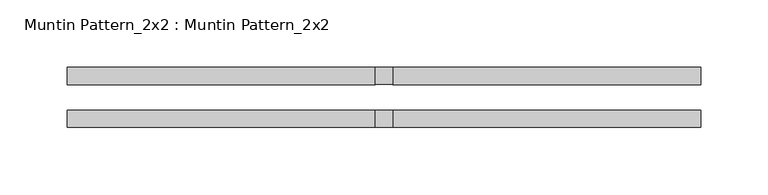
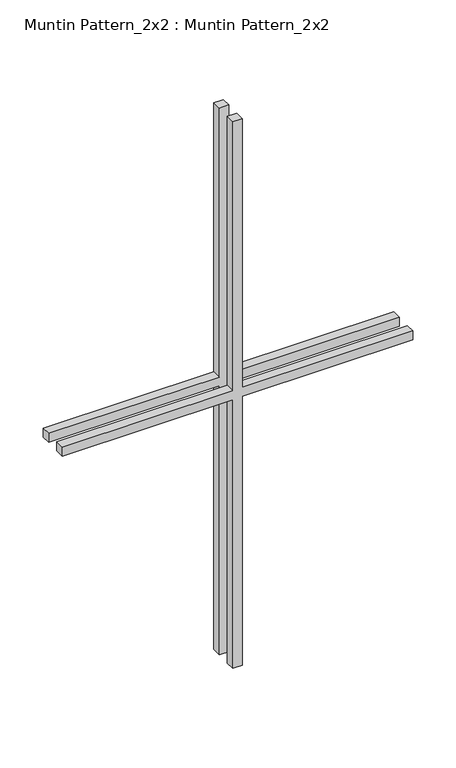
"""IFC4 building model written with IfcOpenShell, lengths in millimetres: proxy geometry, Muntin Pattern_2x2 : Muntin Pattern_2x2."""

from ifc_helpers import new_model, si_unit, frame, origin, place, context, project, spatial, polyline, outline, extrude, source, transform, mapped, element, save


def muntin_pattern_2x2_muntin_pattern_2x2_cf4092f1(model_context):
    return source(origin(), model_context, "Body", "SweptSolid", [
        extrude(outline(polyline([(393.7, -6.35), (393.7, -234.95), (381.0, -234.95), (381.0, -6.35), (0.0, -6.35), (0.0, 6.35), (381.0, 6.35), (381.0, 234.95), (393.7, 234.95), (393.7, 6.35), (774.7, 6.35), (774.7, -6.35), (393.7, -6.35)])), frame((0.0, 9.525, 0.0), z_axis=(0.0, 1.0, 0.0), x_axis=(0.0, 0.0, 1.0)), (0.0, 0.0, 1.0), 12.7),
        extrude(outline(polyline([(393.7, -6.35), (393.7, -234.95), (381.0, -234.95), (381.0, -6.35), (0.0, -6.35), (0.0, 6.35), (381.0, 6.35), (381.0, 234.95), (393.7, 234.95), (393.7, 6.35), (774.7, 6.35), (774.7, -6.35), (393.7, -6.35)])), frame((0.0, -22.225, 0.0), z_axis=(0.0, 1.0, 0.0), x_axis=(0.0, 0.0, 1.0)), (0.0, 0.0, 1.0), 12.7),
    ])


if __name__ == "__main__":
    model = new_model("IFC4")
    model_context = context("Model", 3, world=origin())
    ifc_project = project(units=[si_unit("LENGTHUNIT", "METRE", prefix="MILLI")], contexts=[model_context])
    site = spatial("IfcSite", under=ifc_project)
    building = spatial("IfcBuilding", under=site)
    placement = place(None, origin())
    muntin_pattern_2x2_muntin_pattern_2x2_shape = muntin_pattern_2x2_muntin_pattern_2x2_cf4092f1(model_context)
    element("IfcBuildingElementProxy", 1, Name="Muntin Pattern_2x2 : Muntin Pattern_2x2", ObjectType="Muntin Pattern_2x2 : Muntin Pattern_2x2", at=placement, inside=building, context=model_context, shape_type="MappedRepresentation", body=[
        mapped(muntin_pattern_2x2_muntin_pattern_2x2_shape, transform((0.0, 0.0, 0.0), x_axis=(1.0, 0.0, 0.0), y_axis=(0.0, 1.0, 0.0), z_axis=(0.0, 0.0, 1.0))),
    ])
    save(model, "model.ifc")

# Revit data of these elements
# Type "Muntin Pattern_2x2 : Muntin Pattern_2x2"
#   Width [instance default] = 4' - 0"
#   Thickness = 0' - 0 1/2"
#   Height [instance default] = 4' - 0"
#   Distance = 0' - 0 3/4"
#   Interior Material [instance default] = none
#   Exterior Material [instance default] = none
#   Default Elevation = 0
# Element 1 (IfcBuildingElementProxy, "Muntin Pattern_2x2 : Muntin Pattern_2x2")
#   Width = 1' - 6 1/2"
#   Height = 2' - 6 1/2"
#   Interior Material = Wood - Stained
#   Exterior Material = Clad - White
#   Materials on its faces: "Clad - White", "Wood - Stained"
# Materials
#   "Clad - White": class "Wood", colour RGB 242 242 238, transparency 0, Cost = 0
#   "Wood - Stained": class "Wood", colour RGB 224 178 126, transparency 0, Cost = 0
